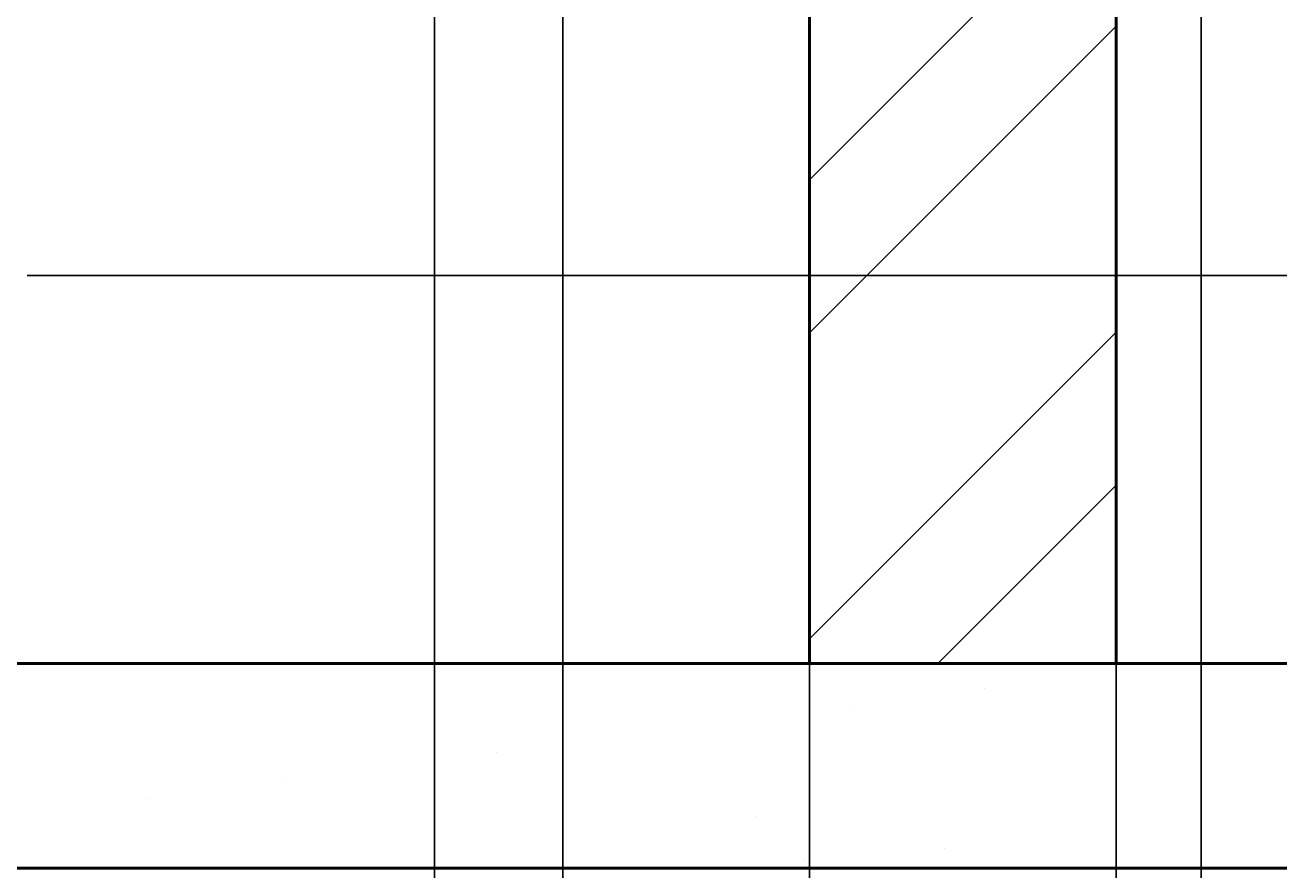
# Model space of a CAD drawing. Units: inches. Extents: x 2812 to 3051, y 1398 to 1659.
# Tile 20 of 65: x 2929 to 2966, y 1410 to 1435. Entities that reach past the tile are written whole.
import ezdxf

# ---------------------------------------------------------------- set-up
doc = ezdxf.new("R2010")
doc.units = ezdxf.units.IN
for name, color, linetype, lineweight in [('A-ANNO-DIMS', 2, 'Continuous', 18), ('S-CONC', 7, 'Continuous', 50), ('S-CONC-PATT', 8, 'Continuous', 18)]:
    doc.layers.add(name, color=color, linetype=linetype, lineweight=lineweight)
doc.styles.get("Standard").update_dxf_attribs({"font": 'arial.ttf'})
doc.dimstyles.get("Standard").update_dxf_attribs({"dimtxt": 0.18, "dimasz": 0.18, "dimexe": 0.18, "dimexo": 0.0625, "dimgap": 0.09, "dimtad": 0, "dimtih": 1, "dimtoh": 1, "dimdec": 4, "dimzin": 0, "dimdsep": 46, "dimtxsty": 'Standard', "dimcen": 0.09, "dimadec": 0, "dimazin": 0, "dimtfac": 1, "dimtdec": 4, "dimtofl": 0, "dimtmove": 0, "dimatfit": 3, "dimfxl": 1, "dimtolj": 1, "dimtzin": 0, "dimarcsym": 0})

# ---------------------------------------------------------------- blocks, each defined once
blk = doc.blocks.new('*D30')
at = {"layer": 'A-ANNO-DIMS', "color": 0, "lineweight": -2, "transparency": 16777216}
for p, q in [((2945.147, 1598.692), (2945.147, 1397.505)), ((2952.385, 1559.757), (2952.385, 1397.505)), ((2945.327, 1397.685), (2948.373, 1397.685)), ((2952.205, 1397.685), (2949.159, 1397.685))]:
    blk.add_line(p, q, dxfattribs=at)
at = {"layer": 'A-ANNO-DIMS', "color": 0, "transparency": 16777216}
for points in [[(2945.327, 1397.715), (2945.327, 1397.655), (2945.147, 1397.685)], [(2952.205, 1397.715), (2952.205, 1397.655), (2952.385, 1397.685)]]:
    blk.add_solid(points, dxfattribs=at)
at = {"layer": 'Defpoints', "color": 0, "transparency": 16777216}
for p in [(2945.147, 1598.754), (2952.385, 1559.82), (2952.385, 1397.685)]:
    blk.add_point(p, dxfattribs=at)
at = {"layer": 'A-ANNO-DIMS', "color": 0, "transparency": 16777216, "insert": (2948.766, 1397.685), "char_height": 0.18, "attachment_point": 5}
blk.add_mtext('\\A1;7.238', dxfattribs=at)
blk = doc.blocks.new('*D31')
at = {"layer": 'A-ANNO-DIMS', "color": 0, "lineweight": -2, "transparency": 16777216}
for p, q in [((2972.272, 1594.192), (2972.272, 1397.505)), ((2961.385, 1559.757), (2961.385, 1397.505)), ((2961.565, 1397.685), (2966.373, 1397.685)), ((2972.092, 1397.685), (2967.283, 1397.685))]:
    blk.add_line(p, q, dxfattribs=at)
at = {"layer": 'A-ANNO-DIMS', "color": 0, "transparency": 16777216}
for points in [[(2961.565, 1397.715), (2961.565, 1397.655), (2961.385, 1397.685)], [(2972.092, 1397.715), (2972.092, 1397.655), (2972.272, 1397.685)]]:
    blk.add_solid(points, dxfattribs=at)
at = {"layer": 'Defpoints', "color": 0, "transparency": 16777216}
for p in [(2972.272, 1594.254), (2961.385, 1559.82), (2972.272, 1397.685)]:
    blk.add_point(p, dxfattribs=at)
at = {"layer": 'A-ANNO-DIMS', "color": 0, "transparency": 16777216, "insert": (2966.828, 1397.685), "char_height": 0.18, "attachment_point": 5}
blk.add_mtext('\\A1;10.887', dxfattribs=at)
blk = doc.blocks.new('*D45')
at = {"layer": 'A-ANNO-DIMS', "color": 0, "lineweight": -2, "transparency": 16777216}
for p, q in [((2896.385, 1487.973), (2896.385, 1397.505)), ((2941.385, 1487.973), (2941.385, 1397.505)), ((2896.565, 1397.685), (2918.662, 1397.685)), ((2941.205, 1397.685), (2919.108, 1397.685))]:
    blk.add_line(p, q, dxfattribs=at)
at = {"layer": 'A-ANNO-DIMS', "color": 0, "transparency": 16777216}
for points in [[(2896.565, 1397.715), (2896.565, 1397.655), (2896.385, 1397.685)], [(2941.205, 1397.715), (2941.205, 1397.655), (2941.385, 1397.685)]]:
    blk.add_solid(points, dxfattribs=at)
at = {"layer": 'Defpoints', "color": 0, "transparency": 16777216}
for p in [(2896.385, 1488.035), (2941.385, 1488.035), (2941.385, 1397.685)]:
    blk.add_point(p, dxfattribs=at)
at = {"layer": 'A-ANNO-DIMS', "color": 0, "transparency": 16777216, "insert": (2918.885, 1397.685), "char_height": 0.18, "attachment_point": 5}
blk.add_mtext('\\A1;45', dxfattribs=at)
blk = doc.blocks.new('*D46')
at = {"layer": 'A-ANNO-DIMS', "color": 0, "lineweight": -2, "transparency": 16777216}
for p, q in [((2941.385, 1487.973), (2941.385, 1397.505)), ((2970.385, 1487.973), (2970.385, 1397.505)), ((2941.565, 1397.685), (2955.664, 1397.685)), ((2970.205, 1397.685), (2956.106, 1397.685))]:
    blk.add_line(p, q, dxfattribs=at)
at = {"layer": 'A-ANNO-DIMS', "color": 0, "transparency": 16777216}
for points in [[(2941.565, 1397.715), (2941.565, 1397.655), (2941.385, 1397.685)], [(2970.205, 1397.715), (2970.205, 1397.655), (2970.385, 1397.685)]]:
    blk.add_solid(points, dxfattribs=at)
at = {"layer": 'Defpoints', "color": 0, "transparency": 16777216}
for p in [(2941.385, 1488.035), (2970.385, 1488.035), (2970.385, 1397.685)]:
    blk.add_point(p, dxfattribs=at)
at = {"layer": 'A-ANNO-DIMS', "color": 0, "transparency": 16777216, "insert": (2955.885, 1397.685), "char_height": 0.18, "attachment_point": 5}
blk.add_mtext('\\A1;29', dxfattribs=at)
blk = doc.blocks.new('*D56')
at = {"layer": 'A-ANNO-DIMS', "color": 0, "lineweight": -2, "transparency": 16777216}
for p, q in [((2880.322, 1452.035), (2811.806, 1452.035)), ((2811.986, 1451.855), (2811.986, 1434.217)), ((2811.986, 1416.215), (2811.986, 1433.853)), ((2952.322, 1416.035), (2811.806, 1416.035))]:
    blk.add_line(p, q, dxfattribs=at)
at = {"layer": 'A-ANNO-DIMS', "color": 0, "transparency": 16777216}
for points in [[(2811.956, 1451.855), (2812.016, 1451.855), (2811.986, 1452.035)], [(2811.956, 1416.215), (2812.016, 1416.215), (2811.986, 1416.035)]]:
    blk.add_solid(points, dxfattribs=at)
at = {"layer": 'Defpoints', "color": 0, "transparency": 16777216}
for p in [(2811.986, 1452.035), (2880.385, 1452.035), (2952.385, 1416.035)]:
    blk.add_point(p, dxfattribs=at)
at = {"layer": 'A-ANNO-DIMS', "color": 0, "transparency": 16777216, "insert": (2811.986, 1434.035), "char_height": 0.18, "attachment_point": 5}
blk.add_mtext('\\A1;36', dxfattribs=at)
blk = doc.blocks.new('*D64')
at = {"layer": 'A-ANNO-DIMS', "color": 0, "lineweight": -2, "transparency": 16777216}
for p, q in [((2929.438, 1427.426), (3051.178, 1427.426)), ((3050.998, 1427.246), (3050.998, 1421.913)), ((3050.998, 1416.215), (3050.998, 1421.549)), ((2952.447, 1416.035), (3051.178, 1416.035))]:
    blk.add_line(p, q, dxfattribs=at)
at = {"layer": 'A-ANNO-DIMS', "color": 0, "transparency": 16777216}
for points in [[(3050.968, 1427.246), (3051.028, 1427.246), (3050.998, 1427.426)], [(3050.968, 1416.215), (3051.028, 1416.215), (3050.998, 1416.035)]]:
    blk.add_solid(points, dxfattribs=at)
at = {"layer": 'Defpoints', "color": 0, "transparency": 16777216}
for p in [(2929.375, 1427.426), (3050.998, 1427.426), (2952.385, 1416.035)]:
    blk.add_point(p, dxfattribs=at)
at = {"layer": 'A-ANNO-DIMS', "color": 0, "transparency": 16777216, "insert": (3050.998, 1421.731), "char_height": 0.18, "attachment_point": 5}
blk.add_mtext('\\A1;11.39', dxfattribs=at)
blk = doc.blocks.new('*D65')
at = {"layer": 'A-ANNO-DIMS', "color": 0, "lineweight": -2, "transparency": 16777216}
for p, q in [((2920.62, 1437.426), (3051.178, 1437.426)), ((3050.998, 1437.246), (3050.998, 1432.608)), ((3050.998, 1427.606), (3050.998, 1432.245)), ((2929.438, 1427.426), (3051.178, 1427.426))]:
    blk.add_line(p, q, dxfattribs=at)
at = {"layer": 'A-ANNO-DIMS', "color": 0, "transparency": 16777216}
for points in [[(3050.968, 1437.246), (3051.028, 1437.246), (3050.998, 1437.426)], [(3050.968, 1427.606), (3051.028, 1427.606), (3050.998, 1427.426)]]:
    blk.add_solid(points, dxfattribs=at)
at = {"layer": 'Defpoints', "color": 0, "transparency": 16777216}
for p in [(2920.558, 1437.426), (3050.998, 1437.426), (2929.375, 1427.426)]:
    blk.add_point(p, dxfattribs=at)
at = {"layer": 'A-ANNO-DIMS', "color": 0, "transparency": 16777216, "insert": (3050.998, 1432.426), "char_height": 0.18, "attachment_point": 5}
blk.add_mtext('\\A1;10', dxfattribs=at)
blk = doc.blocks.new('*D70')
at = {"layer": 'A-ANNO-DIMS', "color": 0, "lineweight": -2, "transparency": 16777216}
for p, q in [((2961.385, 1450.411), (2961.385, 1397.505)), ((2963.874, 1450.411), (2963.874, 1397.505)), ((2961.565, 1397.685), (2962.234, 1397.685)), ((2963.694, 1397.685), (2963.025, 1397.685))]:
    blk.add_line(p, q, dxfattribs=at)
at = {"layer": 'A-ANNO-DIMS', "color": 0, "transparency": 16777216}
for points in [[(2961.565, 1397.715), (2961.565, 1397.655), (2961.385, 1397.685)], [(2963.694, 1397.715), (2963.694, 1397.655), (2963.874, 1397.685)]]:
    blk.add_solid(points, dxfattribs=at)
at = {"layer": 'Defpoints', "color": 0, "transparency": 16777216}
for p in [(2961.385, 1450.474), (2963.874, 1450.474), (2963.874, 1397.685)]:
    blk.add_point(p, dxfattribs=at)
at = {"layer": 'A-ANNO-DIMS', "color": 0, "transparency": 16777216, "insert": (2962.63, 1397.685), "char_height": 0.18, "attachment_point": 5}
blk.add_mtext('\\A1;2.489', dxfattribs=at)
blk = doc.blocks.new('*D75')
at = {"layer": 'A-ANNO-DIMS', "color": 0, "lineweight": -2, "transparency": 16777216}
for p, q in [((2963.812, 1448.474), (2811.806, 1448.474)), ((2811.986, 1448.294), (2811.986, 1432.437)), ((2811.986, 1416.215), (2811.986, 1432.073)), ((2961.322, 1416.035), (2811.806, 1416.035))]:
    blk.add_line(p, q, dxfattribs=at)
at = {"layer": 'A-ANNO-DIMS', "color": 0, "transparency": 16777216}
for points in [[(2811.956, 1448.294), (2812.016, 1448.294), (2811.986, 1448.474)], [(2811.956, 1416.215), (2812.016, 1416.215), (2811.986, 1416.035)]]:
    blk.add_solid(points, dxfattribs=at)
at = {"layer": 'Defpoints', "color": 0, "transparency": 16777216}
for p in [(2811.986, 1448.474), (2963.874, 1448.474), (2961.385, 1416.035)]:
    blk.add_point(p, dxfattribs=at)
at = {"layer": 'A-ANNO-DIMS', "color": 0, "transparency": 16777216, "insert": (2811.986, 1432.255), "char_height": 0.18, "attachment_point": 5}
blk.add_mtext('\\A1;32.44', dxfattribs=at)

msp = doc.modelspace()

# ---------------------------------------------------------------- hatches: boundary and pattern name
at = {"layer": 'S-CONC-PATT'}
h = msp.add_hatch(dxfattribs=at)
h.set_pattern_fill('ANSI32', color=256)
h.paths.add_polyline_path([(3027.3849, 1646.82), (2835.3849, 1646.82), (2835.3849, 1603.2296), (2844.3849, 1603.2296), (2844.3849, 1637.82), (3018.3849, 1637.82), (3018.3849, 1602.5441), (3027.3849, 1602.5441)])
h.paths.add_polyline_path([(2844.3849, 1594.2296), (2835.3849, 1594.2296), (2835.3849, 1550.82), (3027.3849, 1550.82), (3027.3849, 1593.5441), (3018.3849, 1593.5441), (3018.3849, 1559.82), (2844.3849, 1559.82)])
h.paths.add_polyline_path([(2844.3849, 1482.0354), (2835.3849, 1482.0354), (2835.3849, 1463.4959), (2844.3849, 1463.4959)])
h.paths.add_polyline_path([(2844.3849, 1461.4959), (2835.3849, 1461.4959), (2835.3849, 1416.0354), (2844.3849, 1416.0354)])
h.paths.add_polyline_path([(3027.3849, 1482.0354), (3018.3849, 1482.0354), (3018.3849, 1463.2854), (3027.3849, 1463.2854)])
h.paths.add_polyline_path([(3027.3849, 1461.2854), (3018.3849, 1461.2854), (3018.3849, 1416.0354), (3027.3849, 1416.0354)])
h.paths.add_polyline_path([(2961.3849, 1448.4738), (2952.3849, 1448.4738), (2952.3849, 1416.0354), (2961.3849, 1416.0354)])
h.paths.add_polyline_path([(2961.3849, 1462.3026), (2952.3849, 1462.3026), (2952.3849, 1450.4738), (2961.3849, 1450.4738)])
h.paths.add_polyline_path([(2961.3849, 1472.0354), (2952.3849, 1472.0354), (2952.3849, 1462.3026), (2961.3849, 1462.3026)])
h = msp.add_hatch(dxfattribs=at)
h.set_pattern_fill('AR-SAND', color=256, scale=0.3)
h.paths.add_polyline_path([(3036.3849, 1416.0354), (3027.3849, 1416.0354), (2826.3849, 1416.0354), (2826.3849, 1410.0354), (2835.3849, 1410.0354), (3036.3849, 1410.0354)])
h.paths.add_polyline_path([(2970.3849, 1488.0354), (2969.3849, 1488.0354), (2941.3849, 1488.0354), (2941.3849, 1482.0354), (2970.3849, 1482.0354)])
h.paths.add_polyline_path([(3036.3849, 1488.0354), (3035.3849, 1488.0354), (3006.3849, 1488.0354), (3006.3849, 1482.0354), (3027.3849, 1482.0354), (3036.3849, 1482.0354)])
h.paths.add_polyline_path([(3034.3849, 1490.0354), (3008.3849, 1490.0354), (3008.3849, 1489.0354), (3034.3849, 1489.0354)])
h.paths.add_polyline_path([(3035.3849, 1489.0354), (3034.3849, 1489.0354), (3007.3849, 1489.0354), (3007.3849, 1488.0354), (3035.3849, 1488.0354)])
h.paths.add_polyline_path([(2968.3849, 1490.0354), (2943.3849, 1490.0354), (2943.3849, 1489.0354), (2968.3849, 1489.0354)])
h.paths.add_polyline_path([(2969.3849, 1489.0354), (2968.3849, 1489.0354), (2942.3849, 1489.0354), (2942.3849, 1488.0354), (2969.3849, 1488.0354)])
h.paths.add_polyline_path([(2896.3849, 1488.0354), (2826.3849, 1488.0354), (2826.3849, 1482.0354), (2896.3849, 1482.0354)])
h.paths.add_polyline_path([(2895.3849, 1489.0354), (2894.3849, 1489.0354), (2827.3849, 1489.0354), (2827.3849, 1488.0354), (2895.3849, 1488.0354)])
h.paths.add_polyline_path([(2894.3849, 1490.0354), (2828.3849, 1490.0354), (2828.3849, 1489.0354), (2894.3849, 1489.0354)])
h = msp.add_hatch(dxfattribs=at)
h.set_pattern_fill('AR-CONC', color=256, scale=0.3)
h.paths.add_polyline_path([(3036.3849, 1416.0354), (3027.3849, 1416.0354), (2826.3849, 1416.0354), (2826.3849, 1410.0354), (2835.3849, 1410.0354), (3036.3849, 1410.0354)])

# ---------------------------------------------------------------- linework, layer by layer
at = {"layer": 'S-CONC'}
for p, q in [((2952.3849, 1472.0354), (2952.3849, 1416.0354)), ((2961.3849, 1448.4738), (2961.3849, 1416.0354)), ((2826.3849, 1416.0354), (3027.3849, 1416.0354)), ((2835.3849, 1410.0354), (3036.3849, 1410.0354))]:
    msp.add_line(p, q, dxfattribs=at)

# ---------------------------------------------------------------- dimensions: what is measured, and where the dimension line sits
at = {"layer": 'A-ANNO-DIMS'}
for base, p1, p2, override, picture, middle in [((2952.3849, 1397.6854), (2945.1467, 1598.7541), (2952.3849, 1559.82), {"dimdec": 3, "dimlfac": 1, "dimrnd": 0, "dimzin": 0, "dimdsep": 46, "dimlunit": 2}, '*D30', (2948.7658, 1397.6854)), ((2972.2716, 1397.6854), (2961.3849, 1559.82), (2972.2716, 1594.2541), {"dimdec": 3, "dimlfac": 1, "dimrnd": 0, "dimzin": 0, "dimdsep": 46, "dimlunit": 2}, '*D31', (2966.8282, 1397.6854)), ((2941.3849, 1397.6854), (2896.3849, 1488.0354), (2941.3849, 1488.0354), {"dimdec": 0, "dimlfac": 1, "dimrnd": 0, "dimzin": 0, "dimdsep": 46, "dimlunit": 2}, '*D45', (2918.8849, 1397.6854)), ((2970.3849, 1397.6854), (2941.3849, 1488.0354), (2970.3849, 1488.0354), {"dimdec": 0, "dimlfac": 1, "dimrnd": 0, "dimzin": 0, "dimdsep": 46, "dimlunit": 2}, '*D46', (2955.8849, 1397.6854)), ((2963.8741, 1397.6854), (2961.3849, 1450.4738), (2963.8741, 1450.4738), {"dimdec": 3, "dimlfac": 1, "dimrnd": 0, "dimzin": 0, "dimdsep": 46, "dimlunit": 2}, '*D70', (2962.6295, 1397.6854))]:
    dim = msp.add_linear_dim(base=base, p1=p1, p2=p2, dimstyle='Standard', override=override, dxfattribs=at)
    dim.commit()
    dim.dimension.update_dxf_attribs({"geometry": picture, "text_midpoint": middle})
for base, p1, p2, override, picture, middle in [((2811.9855, 1452.0354), (2952.3849, 1416.0354), (2880.3849, 1452.0354), {"dimdec": 0, "dimlfac": 1, "dimrnd": 0, "dimzin": 0, "dimdsep": 46, "dimlunit": 2}, '*D56', (2811.9855, 1434.0354)), ((2811.9855, 1448.4738), (2961.3849, 1416.0354), (2963.8741, 1448.4738), {"dimdec": 2, "dimlfac": 1, "dimrnd": 0, "dimzin": 0, "dimdsep": 46, "dimlunit": 2}, '*D75', (2811.9855, 1432.2546)), ((3050.998, 1437.4265), (2929.3751, 1427.4265), (2920.5577, 1437.4265), {"dimdec": 0, "dimlfac": 1, "dimrnd": 0, "dimzin": 0, "dimdsep": 46, "dimlunit": 2}, '*D65', (3050.998, 1432.4265)), ((3050.998, 1427.4265), (2952.3849, 1416.0354), (2929.3751, 1427.4265), {"dimdec": 2, "dimlfac": 1, "dimrnd": 0, "dimzin": 0, "dimdsep": 46, "dimlunit": 2}, '*D64', (3050.998, 1421.7309))]:
    dim = msp.add_linear_dim(base=base, p1=p1, p2=p2, angle=90, dimstyle='Standard', override=override, dxfattribs=at)
    dim.commit()
    dim.dimension.update_dxf_attribs({"geometry": picture, "text_midpoint": middle})

doc.saveas('drawing.dxf')
